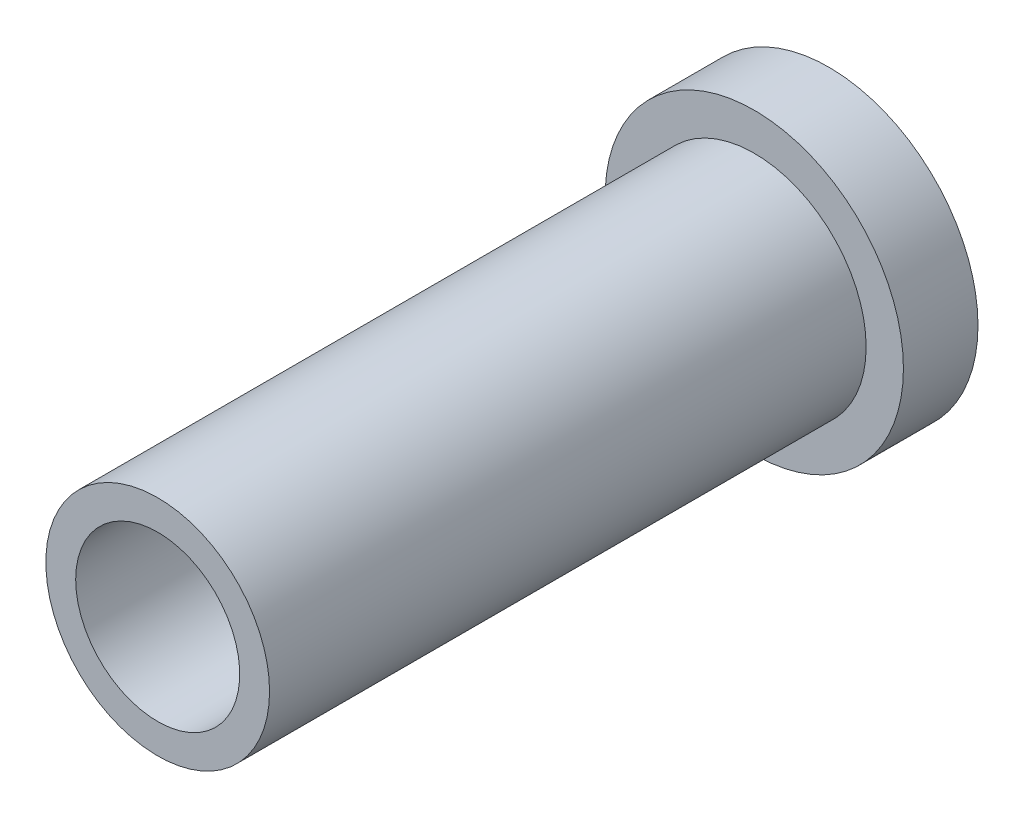
ISO-10303-21;
HEADER;
FILE_DESCRIPTION(('STEP AP214'),'2;1');
FILE_NAME('part.step','',(''),(''),'','','');
FILE_SCHEMA(('AUTOMOTIVE_DESIGN { 1 0 10303 214 1 1 1 1 }'));
ENDSEC;
DATA;
#1=APPLICATION_CONTEXT('core data for automotive mechanical design processes');
#2=APPLICATION_PROTOCOL_DEFINITION('international standard','automotive_design',2000,#1);
#3=PRODUCT_CONTEXT('',#1,'mechanical');
#4=PRODUCT('Part','Part','',(#3));
#5=PRODUCT_RELATED_PRODUCT_CATEGORY('part','',(#4));
#6=PRODUCT_DEFINITION_FORMATION('','',#4);
#7=PRODUCT_DEFINITION_CONTEXT('part definition',#1,'design');
#8=PRODUCT_DEFINITION('design','',#6,#7);
#9=PRODUCT_DEFINITION_SHAPE('','',#8);
#10=(LENGTH_UNIT() NAMED_UNIT(*) SI_UNIT(.MILLI.,.METRE.));
#11=(NAMED_UNIT(*) PLANE_ANGLE_UNIT() SI_UNIT($,.RADIAN.));
#12=(NAMED_UNIT(*) SI_UNIT($,.STERADIAN.) SOLID_ANGLE_UNIT());
#13=UNCERTAINTY_MEASURE_WITH_UNIT(LENGTH_MEASURE(1.E-05),#10,'distance_accuracy_value','');
#14=(GEOMETRIC_REPRESENTATION_CONTEXT(3) GLOBAL_UNCERTAINTY_ASSIGNED_CONTEXT((#13)) GLOBAL_UNIT_ASSIGNED_CONTEXT((#10,
#11,#12)) REPRESENTATION_CONTEXT('',''));
#15=CARTESIAN_POINT('',(0.,0.,0.));
#16=DIRECTION('',(0.,0.,1.));
#17=DIRECTION('',(1.,0.,0.));
#18=AXIS2_PLACEMENT_3D('',#15,#16,#17);
#19=CARTESIAN_POINT('',(0.,0.,5.));
#20=DIRECTION('',(0.,0.,-1.));
#21=DIRECTION('',(-1.,0.,0.));
#22=AXIS2_PLACEMENT_3D('',#19,#20,#21);
#23=CYLINDRICAL_SURFACE('',#22,10.);
#24=CARTESIAN_POINT('',(0.,0.,5.));
#25=DIRECTION('',(0.,0.,1.));
#26=DIRECTION('',(1.,0.,0.));
#27=AXIS2_PLACEMENT_3D('',#24,#25,#26);
#28=CIRCLE('',#27,10.);
#29=CARTESIAN_POINT('',(10.,0.,5.));
#30=VERTEX_POINT('',#29);
#31=EDGE_CURVE('E42',#30,#30,#28,.T.);
#32=ORIENTED_EDGE('',*,*,#31,.F.);
#33=EDGE_LOOP('',(#32));
#34=FACE_BOUND('',#33,.T.);
#35=CARTESIAN_POINT('',(0.,0.,0.));
#36=DIRECTION('',(0.,0.,1.));
#37=DIRECTION('',(1.,0.,0.));
#38=AXIS2_PLACEMENT_3D('',#35,#36,#37);
#39=CIRCLE('',#38,10.);
#40=CARTESIAN_POINT('',(10.,0.,0.));
#41=VERTEX_POINT('',#40);
#42=EDGE_CURVE('E37',#41,#41,#39,.T.);
#43=ORIENTED_EDGE('',*,*,#42,.T.);
#44=EDGE_LOOP('',(#43));
#45=FACE_BOUND('',#44,.T.);
#46=ADVANCED_FACE('F40',(#34,#45),#23,.T.);
#47=CARTESIAN_POINT('',(0.,0.,5.));
#48=DIRECTION('',(0.,0.,1.));
#49=DIRECTION('',(1.,0.,0.));
#50=AXIS2_PLACEMENT_3D('',#47,#48,#49);
#51=PLANE('',#50);
#52=CARTESIAN_POINT('',(0.,0.,5.));
#53=DIRECTION('',(0.,0.,1.));
#54=DIRECTION('',(1.,0.,0.));
#55=AXIS2_PLACEMENT_3D('',#52,#53,#54);
#56=CIRCLE('',#55,7.5);
#57=CARTESIAN_POINT('',(7.5,0.,5.));
#58=VERTEX_POINT('',#57);
#59=EDGE_CURVE('E10',#58,#58,#56,.T.);
#60=ORIENTED_EDGE('',*,*,#59,.F.);
#61=EDGE_LOOP('',(#60));
#62=FACE_BOUND('',#61,.T.);
#63=ORIENTED_EDGE('',*,*,#31,.T.);
#64=EDGE_LOOP('',(#63));
#65=FACE_BOUND('',#64,.T.);
#66=ADVANCED_FACE('F71',(#62,#65),#51,.T.);
#67=CARTESIAN_POINT('',(0.,0.,0.));
#68=DIRECTION('',(0.,0.,1.));
#69=DIRECTION('',(1.,0.,0.));
#70=AXIS2_PLACEMENT_3D('',#67,#68,#69);
#71=PLANE('',#70);
#72=CARTESIAN_POINT('',(0.,0.,0.));
#73=DIRECTION('',(0.,0.,-1.));
#74=DIRECTION('',(-1.,0.,0.));
#75=AXIS2_PLACEMENT_3D('',#72,#73,#74);
#76=CIRCLE('',#75,5.5);
#77=CARTESIAN_POINT('',(-5.5,0.,0.));
#78=VERTEX_POINT('',#77);
#79=EDGE_CURVE('E53',#78,#78,#76,.T.);
#80=ORIENTED_EDGE('',*,*,#79,.F.);
#81=EDGE_LOOP('',(#80));
#82=FACE_BOUND('',#81,.T.);
#83=ORIENTED_EDGE('',*,*,#42,.F.);
#84=EDGE_LOOP('',(#83));
#85=FACE_BOUND('',#84,.T.);
#86=ADVANCED_FACE('F69',(#82,#85),#71,.F.);
#87=CARTESIAN_POINT('',(0.,0.,45.));
#88=DIRECTION('',(0.,0.,-1.));
#89=DIRECTION('',(-1.,0.,0.));
#90=AXIS2_PLACEMENT_3D('',#87,#88,#89);
#91=CYLINDRICAL_SURFACE('',#90,7.5);
#92=CARTESIAN_POINT('',(0.,0.,45.));
#93=DIRECTION('',(0.,0.,1.));
#94=DIRECTION('',(1.,0.,0.));
#95=AXIS2_PLACEMENT_3D('',#92,#93,#94);
#96=CIRCLE('',#95,7.5);
#97=CARTESIAN_POINT('',(7.5,0.,45.));
#98=VERTEX_POINT('',#97);
#99=EDGE_CURVE('E49',#98,#98,#96,.T.);
#100=ORIENTED_EDGE('',*,*,#99,.F.);
#101=EDGE_LOOP('',(#100));
#102=FACE_BOUND('',#101,.T.);
#103=ORIENTED_EDGE('',*,*,#59,.T.);
#104=EDGE_LOOP('',(#103));
#105=FACE_BOUND('',#104,.T.);
#106=ADVANCED_FACE('F75',(#102,#105),#91,.T.);
#107=CARTESIAN_POINT('',(0.,0.,45.));
#108=DIRECTION('',(0.,0.,1.));
#109=DIRECTION('',(1.,0.,0.));
#110=AXIS2_PLACEMENT_3D('',#107,#108,#109);
#111=PLANE('',#110);
#112=CARTESIAN_POINT('',(0.,0.,45.));
#113=DIRECTION('',(0.,0.,-1.));
#114=DIRECTION('',(-1.,0.,0.));
#115=AXIS2_PLACEMENT_3D('',#112,#113,#114);
#116=CIRCLE('',#115,5.5);
#117=CARTESIAN_POINT('',(-5.5,0.,45.));
#118=VERTEX_POINT('',#117);
#119=EDGE_CURVE('E52',#118,#118,#116,.T.);
#120=ORIENTED_EDGE('',*,*,#119,.T.);
#121=EDGE_LOOP('',(#120));
#122=FACE_BOUND('',#121,.T.);
#123=ORIENTED_EDGE('',*,*,#99,.T.);
#124=EDGE_LOOP('',(#123));
#125=FACE_BOUND('',#124,.T.);
#126=ADVANCED_FACE('F58',(#122,#125),#111,.T.);
#127=CARTESIAN_POINT('',(0.,0.,45.));
#128=DIRECTION('',(0.,0.,-1.));
#129=DIRECTION('',(-1.,0.,0.));
#130=AXIS2_PLACEMENT_3D('',#127,#128,#129);
#131=CYLINDRICAL_SURFACE('',#130,5.5);
#132=CARTESIAN_POINT('',(-5.5,0.,45.));
#133=CARTESIAN_POINT('',(-5.5,0.,44.53125));
#134=CARTESIAN_POINT('',(-5.5,0.,44.0625));
#135=CARTESIAN_POINT('',(-5.5,0.,43.125));
#136=CARTESIAN_POINT('',(-5.5,0.,42.65625));
#137=CARTESIAN_POINT('',(-5.5,0.,41.71875));
#138=CARTESIAN_POINT('',(-5.5,0.,41.25));
#139=CARTESIAN_POINT('',(-5.5,0.,40.3125));
#140=CARTESIAN_POINT('',(-5.5,0.,39.84375));
#141=CARTESIAN_POINT('',(-5.5,0.,38.90625));
#142=CARTESIAN_POINT('',(-5.5,0.,38.4375));
#143=CARTESIAN_POINT('',(-5.5,0.,37.5));
#144=CARTESIAN_POINT('',(-5.5,0.,37.03125));
#145=CARTESIAN_POINT('',(-5.5,0.,36.09375));
#146=CARTESIAN_POINT('',(-5.5,0.,35.625));
#147=CARTESIAN_POINT('',(-5.5,0.,34.6875));
#148=CARTESIAN_POINT('',(-5.5,0.,34.21875));
#149=CARTESIAN_POINT('',(-5.5,0.,33.28125));
#150=CARTESIAN_POINT('',(-5.5,0.,32.8125));
#151=CARTESIAN_POINT('',(-5.5,0.,31.875));
#152=CARTESIAN_POINT('',(-5.5,0.,31.40625));
#153=CARTESIAN_POINT('',(-5.5,0.,30.46875));
#154=CARTESIAN_POINT('',(-5.5,0.,30.));
#155=CARTESIAN_POINT('',(-5.5,0.,29.0625));
#156=CARTESIAN_POINT('',(-5.5,0.,28.59375));
#157=CARTESIAN_POINT('',(-5.5,0.,27.65625));
#158=CARTESIAN_POINT('',(-5.5,0.,27.1875));
#159=CARTESIAN_POINT('',(-5.5,0.,26.25));
#160=CARTESIAN_POINT('',(-5.5,0.,25.78125));
#161=CARTESIAN_POINT('',(-5.5,0.,24.84375));
#162=CARTESIAN_POINT('',(-5.5,0.,24.375));
#163=CARTESIAN_POINT('',(-5.5,0.,23.4375));
#164=CARTESIAN_POINT('',(-5.5,0.,22.96875));
#165=CARTESIAN_POINT('',(-5.5,0.,22.03125));
#166=CARTESIAN_POINT('',(-5.5,0.,21.5625));
#167=CARTESIAN_POINT('',(-5.5,0.,20.625));
#168=CARTESIAN_POINT('',(-5.5,0.,20.15625));
#169=CARTESIAN_POINT('',(-5.5,0.,19.21875));
#170=CARTESIAN_POINT('',(-5.5,0.,18.75));
#171=CARTESIAN_POINT('',(-5.5,0.,17.8125));
#172=CARTESIAN_POINT('',(-5.5,0.,17.34375));
#173=CARTESIAN_POINT('',(-5.5,0.,16.40625));
#174=CARTESIAN_POINT('',(-5.5,0.,15.9375));
#175=CARTESIAN_POINT('',(-5.5,0.,15.));
#176=CARTESIAN_POINT('',(-5.5,0.,14.53125));
#177=CARTESIAN_POINT('',(-5.5,0.,13.59375));
#178=CARTESIAN_POINT('',(-5.5,0.,13.125));
#179=CARTESIAN_POINT('',(-5.5,0.,12.1875));
#180=CARTESIAN_POINT('',(-5.5,0.,11.71875));
#181=CARTESIAN_POINT('',(-5.5,0.,10.78125));
#182=CARTESIAN_POINT('',(-5.5,0.,10.3125));
#183=CARTESIAN_POINT('',(-5.5,0.,9.37500000000001));
#184=CARTESIAN_POINT('',(-5.5,0.,8.90625000000001));
#185=CARTESIAN_POINT('',(-5.5,0.,7.96875000000001));
#186=CARTESIAN_POINT('',(-5.5,0.,7.50000000000001));
#187=CARTESIAN_POINT('',(-5.5,0.,6.56250000000001));
#188=CARTESIAN_POINT('',(-5.5,0.,6.09375000000001));
#189=CARTESIAN_POINT('',(-5.5,0.,5.15625000000001));
#190=CARTESIAN_POINT('',(-5.5,0.,4.68750000000001));
#191=CARTESIAN_POINT('',(-5.5,0.,3.75000000000001));
#192=CARTESIAN_POINT('',(-5.5,0.,3.28125000000001));
#193=CARTESIAN_POINT('',(-5.5,0.,2.34375000000001));
#194=CARTESIAN_POINT('',(-5.5,0.,1.87500000000001));
#195=CARTESIAN_POINT('',(-5.5,0.,0.937500000000006));
#196=CARTESIAN_POINT('',(-5.5,0.,0.468750000000007));
#197=CARTESIAN_POINT('',(-5.5,0.,0.));
#198=B_SPLINE_CURVE_WITH_KNOTS('',3,(#132,#133,#134,#135,#136,#137,#138,#139,#140,#141,#142,
#143,#144,#145,#146,#147,#148,#149,#150,#151,#152,#153,#154,#155,#156,#157,#158,#159,#160,#161,
#162,#163,#164,#165,#166,#167,#168,#169,#170,#171,#172,#173,#174,#175,#176,#177,#178,#179,#180,
#181,#182,#183,#184,#185,#186,#187,#188,#189,#190,#191,#192,#193,#194,#195,#196,#197),
.UNSPECIFIED.,.F.,.F.,(4,2,2,2,2,2,2,2,2,2,2,2,2,2,2,2,2,2,2,2,2,2,2,2,2,2,2,2,2,2,2,2,4),(0.,
1.40625,2.8125,4.21875,5.62500000000001,7.03125,8.4375,9.84375000000001,11.25,12.65625,14.0625,
15.46875,16.875,18.28125,19.6875,21.09375,22.5,23.90625,25.3125,26.71875,28.125,29.53125,
30.9375,32.34375,33.75,35.15625,36.5625,37.96875,39.375,40.78125,42.1875,43.59375,45.),.UNSPECIFIED.);
#199=EDGE_CURVE('BSEAM62',#118,#78,#198,.T.);
#200=ORIENTED_EDGE('',*,*,#119,.F.);
#201=ORIENTED_EDGE('',*,*,#79,.T.);
#202=ORIENTED_EDGE('',*,*,#199,.T.);
#203=ORIENTED_EDGE('',*,*,#199,.F.);
#204=EDGE_LOOP('',(#200,#202,#201,#203));
#205=FACE_BOUND('',#204,.T.);
#206=ADVANCED_FACE('F62',(#205),#131,.F.);
#207=CLOSED_SHELL('',(#46,#66,#86,#106,#126,#206));
#208=MANIFOLD_SOLID_BREP('B2',#207);
#209=ADVANCED_BREP_SHAPE_REPRESENTATION('',(#18,#208),#14);
#210=SHAPE_DEFINITION_REPRESENTATION(#9,#209);
ENDSEC;
END-ISO-10303-21;
